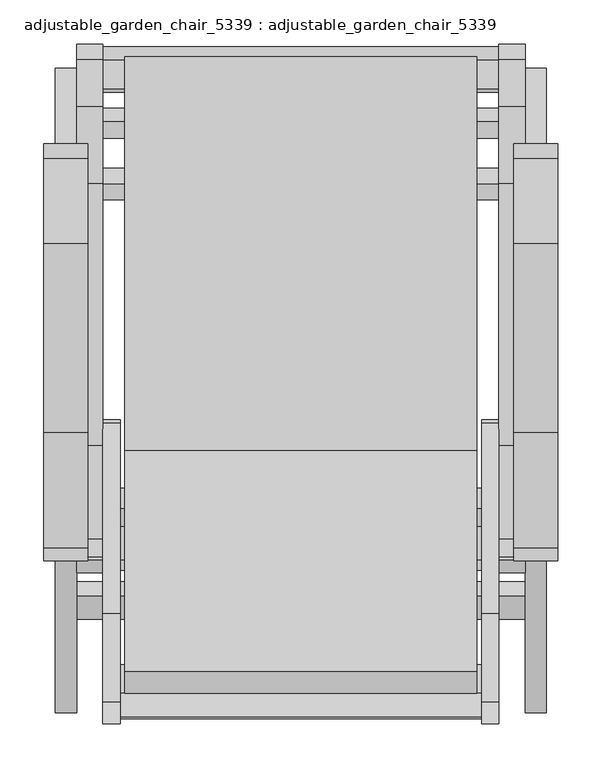
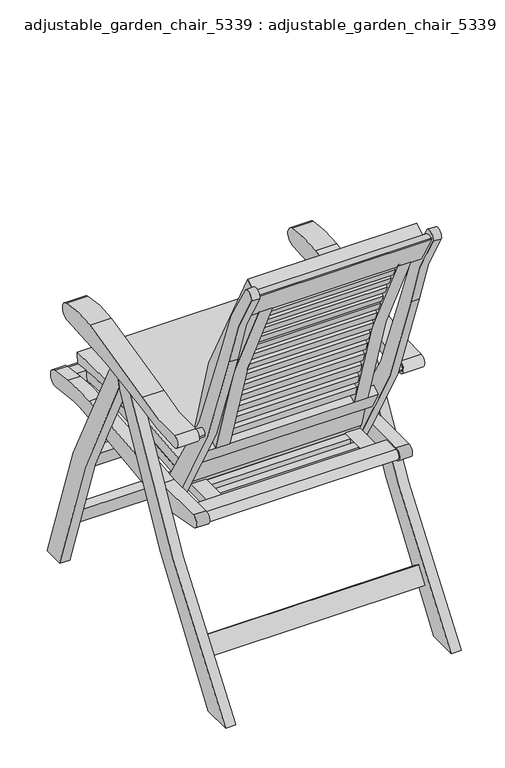
"""IFC4 building model written with IfcOpenShell, lengths in millimetres: furniture geometry, adjustable_garden_chair_5339 : adjustable_garden_chair_5339."""

from ifc_helpers import new_model, si_unit, point, frame, frame_2d, origin, place, context, project, spatial, polyline, circle_curve, trimmed, segment, composite_curve, outline, extrude, source, transform, mapped, element, save


def adjustable_garden_chair_5339_adjustable_garden_chair_5339_fbaf4b35(model_context):
    return source(origin(), model_context, "Body", "SweptSolid", [
        extrude(outline(composite_curve([segment(trimmed(circle_curve(frame_2d((343.645132, -510.0114028)), 1212.8355828), [point((-43.4212159, 639.4014009))], [point((170.6132595, 690.417738))], False, "CARTESIAN"), True, "CONTINUOUS"), segment(trimmed(circle_curve(frame_2d((209.9588085, 417.4533248)), 275.7855019), [point((170.6132595, 690.417738))], [point((267.5231892, 687.1642537))], False, "CARTESIAN"), True, "CONTINUOUS"), segment(trimmed(circle_curve(frame_2d((263.0738268, 666.3173055)), 21.3164742), [point((267.5231892, 687.1642537))], [point((263.2618422, 645.0016605))], False, "CARTESIAN"), True, "CONTINUOUS"), segment(trimmed(circle_curve(frame_2d((275.8190799, -778.6351578)), 1423.692198), [point((263.2618422, 645.0016605))], [point((-39.8991519, 609.6088672))], True, "CARTESIAN"), True, "CONTINUOUS"), segment(trimmed(circle_curve(frame_2d((-181.4513875, 1232.0279279)), 638.3122454), [point((-39.8991519, 609.6088672))], [point((-173.9655536, 593.7595793))], False, "CARTESIAN"), True, "CONTINUOUS"), segment(trimmed(circle_curve(frame_2d((-174.7344479, 608.5698693)), 14.8302356), [point((-173.9655536, 593.7595793))], [point((-175.5033422, 623.3801593))], False, "CARTESIAN"), True, "CONTINUOUS"), segment(trimmed(circle_curve(frame_2d((-148.1612086, 950.4320275)), 328.1928043), [point((-175.5033422, 623.3801593))], [point((-43.4212159, 639.4014009))], True, "CARTESIAN"), True, "CONTINUOUS")], self_intersect=False)), frame((242.0, 0.0, 0.0), z_axis=(1.0, 0.0, 0.0), x_axis=(0.0, 1.0, 0.0)), (0.0, 0.0, 1.0), 50.0),
        extrude(outline(composite_curve([segment(trimmed(circle_curve(frame_2d((343.645132, -510.0114028)), 1212.8355828), [point((-43.4212159, 639.4014009))], [point((170.6132595, 690.417738))], False, "CARTESIAN"), True, "CONTINUOUS"), segment(trimmed(circle_curve(frame_2d((209.9588085, 417.4533248)), 275.7855019), [point((170.6132595, 690.417738))], [point((267.5231892, 687.1642537))], False, "CARTESIAN"), True, "CONTINUOUS"), segment(trimmed(circle_curve(frame_2d((263.0738268, 666.3173055)), 21.3164742), [point((267.5231892, 687.1642537))], [point((263.2618422, 645.0016605))], False, "CARTESIAN"), True, "CONTINUOUS"), segment(trimmed(circle_curve(frame_2d((275.8190799, -778.6351578)), 1423.692198), [point((263.2618422, 645.0016605))], [point((-39.8991519, 609.6088672))], True, "CARTESIAN"), True, "CONTINUOUS"), segment(trimmed(circle_curve(frame_2d((-181.4513875, 1232.0279279)), 638.3122454), [point((-39.8991519, 609.6088672))], [point((-173.9655536, 593.7595793))], False, "CARTESIAN"), True, "CONTINUOUS"), segment(trimmed(circle_curve(frame_2d((-174.7344479, 608.5698693)), 14.8302356), [point((-173.9655536, 593.7595793))], [point((-175.5033422, 623.3801593))], False, "CARTESIAN"), True, "CONTINUOUS"), segment(trimmed(circle_curve(frame_2d((-148.1612086, 950.4320275)), 328.1928043), [point((-175.5033422, 623.3801593))], [point((-43.4212159, 639.4014009))], True, "CARTESIAN"), True, "CONTINUOUS")], self_intersect=False)), frame((-292.0, 0.0, 0.0), z_axis=(1.0, 0.0, 0.0), x_axis=(0.0, 1.0, 0.0)), (0.0, 0.0, 1.0), 50.0),
        extrude(outline(polyline([(0.0, 20.0), (295.0, 20.0), (295.0, 0.0), (0.0, 0.0), (0.0, 20.0)])), frame((147.5, -137.5882722, 568.6800749), z_axis=(0.0, -0.2533030270582979, 0.9673869838296892), x_axis=(-1.0, 0.0, 0.0)), (0.0, 0.0, 1.0), 20.0),
        extrude(outline(polyline([(0.0, 20.0), (295.0, 20.0), (295.0, 0.0), (0.0, 0.0), (0.0, 20.0)])), frame((147.5, -147.2074959, 603.5678435), z_axis=(0.0, -0.2719015325291372, 0.9623250784471465), x_axis=(-1.0, 0.0, 0.0)), (0.0, 0.0, 1.0), 20.0),
        extrude(outline(polyline([(0.0, 19.9999999), (295.0, 19.9999999), (295.0, 0.0), (0.0, 0.0), (0.0, 19.9999999)])), frame((147.5, -157.4973647, 638.2637288), z_axis=(0.0, -0.2903990191599495, 0.9569056430343272), x_axis=(-1.0, 0.0, 0.0)), (0.0, 0.0, 1.0), 20.0),
        extrude(outline(polyline([(0.0, 20.0000001), (295.0, 20.0000001), (295.0, 0.0), (0.0, 0.0), (0.0, 20.0000001)])), frame((147.5, -168.4540556, 672.7548405), z_axis=(0.0, -0.30878861462961876, 0.9511306910593943), x_axis=(-1.0, 0.0, 0.0)), (0.0, 0.0, 1.0), 20.0),
        extrude(outline(polyline([(0.0, 20.0), (295.0, 20.0), (295.0, 0.0), (0.0, 0.0), (0.0, 20.0)])), frame((147.5, -180.073498, 707.028364), z_axis=(0.0, -0.3270634867015429, 0.9450023680746149), x_axis=(-1.0, 0.0, 0.0)), (0.0, 0.0, 1.0), 20.0),
        extrude(outline(polyline([(0.0, 20.0), (295.0, 20.0), (295.0, 0.0), (0.0, 0.0), (0.0, 20.0)])), frame((147.5, -192.3513749, 741.071566), z_axis=(0.0, -0.3452168457619835, 0.9385229509192341), x_axis=(-1.0, 0.0, 0.0)), (0.0, 0.0, 1.0), 20.0),
        extrude(outline(polyline([(0.0, 20.0), (295.0, 20.0), (295.0, 0.0), (0.0, 0.0), (0.0, 20.0)])), frame((147.5, -205.2831247, 774.8717983), z_axis=(0.0, -0.3632419473426192, 0.9316948468735576), x_axis=(-1.0, 0.0, 0.0)), (0.0, 0.0, 1.0), 20.0),
        extrude(outline(polyline([(0.0, 20.0), (295.0, 20.0), (295.0, 0.0), (0.0, 0.0), (0.0, 20.0)])), frame((147.5, -218.863943, 808.4165033), z_axis=(0.0, -0.38113209462627146, 0.9245205927645911), x_axis=(-1.0, 0.0, 0.0)), (0.0, 0.0, 1.0), 20.0),
        extrude(outline(polyline([(0.0, 20.0000001), (295.0, 20.0000001), (295.0, 0.0), (0.0, 0.0), (0.0, 20.0000001)])), frame((147.5, -233.088784, 841.6932183), z_axis=(0.0, -0.39888064093497316, 0.9170028540235331), x_axis=(-1.0, 0.0, 0.0)), (0.0, 0.0, 1.0), 20.0),
        extrude(outline(polyline([(0.0, 20.0), (295.0, 20.0), (295.0, 0.0), (0.0, 0.0), (0.0, 20.0)])), frame((147.5, -244.4121321, 867.0975304), z_axis=(0.0, -0.4164809921993657, 0.9091444236955051), x_axis=(-1.0, 0.0, 0.0)), (0.0, 0.0, 1.0), 20.0),
        extrude(outline(polyline([(0.0, 20.0), (295.0, 20.0), (295.0, 0.0), (0.0, 0.0), (0.0, 20.0)])), frame((147.5, -259.9089267, 899.8012797), z_axis=(0.0, -0.43392660940863675, 0.9009482214018321), x_axis=(-1.0, 0.0, 0.0)), (0.0, 0.0, 1.0), 20.0),
        extrude(outline(polyline([(0.0, 20.0000001), (295.0, 20.0000001), (295.0, 0.0), (0.0, 0.0), (0.0, 20.0000001)])), frame((147.5, -276.0331794, 932.2002663), z_axis=(0.0, -0.4512110110398427, 0.892417292255368), x_axis=(-1.0, 0.0, 0.0)), (0.0, 0.0, 1.0), 20.0),
        extrude(outline(polyline([(0.0, 20.0), (295.0, 20.0), (295.0, 0.0), (0.0, 0.0), (0.0, 20.0)])), frame((147.5, -292.7788997, 964.2824531), z_axis=(0.0, -0.4683277754660565, 0.8835548057291156), x_axis=(-1.0, 0.0, 0.0)), (0.0, 0.0, 1.0), 20.0),
        extrude(outline(composite_curve([segment(trimmed(circle_curve(frame_2d((-1820.3447932, 139.3902819)), 1716.607402), [point((-150.6635772, 538.0199468))], [point((-330.8196286, 992.6521155))], True, "CARTESIAN"), True, "CONTINUOUS"), segment(polyline([(-330.8196286, 992.6521155), (-311.3178699, 1002.7482844)]), True, "CONTINUOUS"), segment(trimmed(circle_curve(frame_2d((-1820.3447932, 139.3902819)), 1738.5480424), [point((-311.3178699, 1002.7482844))], [point((-130.6557697, 548.6582867))], False, "CARTESIAN"), True, "CONTINUOUS"), segment(polyline([(-130.6557697, 548.6582867), (-150.6635772, 538.0199468)]), True, "CONTINUOUS")], self_intersect=False)), frame((147.5, 0.0, 0.0), z_axis=(1.0, 0.0, 0.0), x_axis=(0.0, 1.0, 0.0)), (0.0, 0.0, 1.0), 32.5),
        extrude(outline(composite_curve([segment(trimmed(circle_curve(frame_2d((-1820.3447932, 139.3902819)), 1716.607402), [point((-150.6635772, 538.0199468))], [point((-330.8196286, 992.6521155))], True, "CARTESIAN"), True, "CONTINUOUS"), segment(polyline([(-330.8196286, 992.6521155), (-311.3178699, 1002.7482844)]), True, "CONTINUOUS"), segment(trimmed(circle_curve(frame_2d((-1820.3447932, 139.3902819)), 1738.5480424), [point((-311.3178699, 1002.7482844))], [point((-130.6557697, 548.6582867))], False, "CARTESIAN"), True, "CONTINUOUS"), segment(polyline([(-130.6557697, 548.6582867), (-150.6635772, 538.0199468)]), True, "CONTINUOUS")], self_intersect=False)), frame((-180.0, 0.0, 0.0), z_axis=(1.0, 0.0, 0.0), x_axis=(0.0, 1.0, 0.0)), (0.0, 0.0, 1.0), 32.5),
        extrude(outline(polyline([(0.0, 22.0), (411.0, 22.0), (411.0, 0.0), (0.0, 0.0), (0.0, 22.0)])), frame((205.5, -107.1821916, 504.5109071), z_axis=(0.0, -0.46947156278588487, 0.8829475928589302), x_axis=(-1.0, 0.0, 0.0)), (0.0, 0.0, 1.0), 50.0),
        extrude(outline(composite_curve([segment(polyline([(-369.2008252, 1058.8126612), (-367.4620723, 1059.800962)]), True, "CONTINUOUS"), segment(trimmed(circle_curve(frame_2d((-357.5790638, 1042.4134336)), 20.0), [point((-367.4620723, 1059.800962))], [point((-340.1915354, 1052.2964421))], False, "CARTESIAN"), True, "CONTINUOUS"), segment(polyline([(-340.1915354, 1052.2964421), (-308.0717579, 995.7869748), (-327.1980391, 984.9156655), (-369.2008252, 1058.8126612)]), True, "CONTINUOUS")], self_intersect=False)), frame((-205.5, 0.0, 0.0), z_axis=(1.0, 0.0, 0.0), x_axis=(0.0, 1.0, 0.0)), (0.0, 0.0, 1.0), 411.0),
        extrude(outline(composite_curve([segment(trimmed(circle_curve(frame_2d((-878.1941568, 714.0152031)), 609.3375862), [point((-284.5644955, 851.478359))], [point((-374.7410315, 1057.2749365))], True, "CARTESIAN"), True, "CONTINUOUS"), segment(trimmed(circle_curve(frame_2d((-359.5368178, 1059.9113552)), 15.4310991), [point((-374.7410315, 1057.2749365))], [point((-350.3591165, 1072.3165403))], False, "CARTESIAN"), True, "CONTINUOUS"), segment(trimmed(circle_curve(frame_2d((-939.3593126, 662.5924291)), 717.4922148), [point((-350.3591165, 1072.3165403))], [point((-249.8732333, 861.0968995))], False, "CARTESIAN"), True, "CONTINUOUS"), segment(trimmed(circle_curve(frame_2d((1197.5178376, 1277.8037867)), 1506.1824398), [point((-249.8732333, 861.0968995))], [point((-33.307137, 409.6704883))], True, "CARTESIAN"), True, "CONTINUOUS"), segment(trimmed(circle_curve(frame_2d((-52.4582417, 396.9808098)), 22.9737405), [point((-33.307137, 409.6704883))], [point((-71.610087, 384.292249))], False, "CARTESIAN"), True, "CONTINUOUS"), segment(trimmed(circle_curve(frame_2d((1314.5285091, 1298.2546646)), 1660.3335522), [point((-71.610087, 384.292249))], [point((-284.5644955, 851.478359))], False, "CARTESIAN"), True, "CONTINUOUS")], self_intersect=False)), frame((205.5, 0.0, 0.0), z_axis=(1.0, 0.0, 0.0), x_axis=(0.0, 1.0, 0.0)), (0.0, 0.0, 1.0), 19.5),
        extrude(outline(composite_curve([segment(trimmed(circle_curve(frame_2d((-878.1941568, 714.0152031)), 609.3375862), [point((-284.5644955, 851.478359))], [point((-374.7410315, 1057.2749365))], True, "CARTESIAN"), True, "CONTINUOUS"), segment(trimmed(circle_curve(frame_2d((-359.53684, 1059.9114029)), 15.4310853), [point((-374.7410315, 1057.2749365))], [point((-350.3591359, 1072.3165688))], False, "CARTESIAN"), True, "CONTINUOUS"), segment(trimmed(circle_curve(frame_2d((-939.3594209, 662.5923787)), 717.4923328), [point((-350.3591359, 1072.3165688))], [point((-249.8732333, 861.0968995))], False, "CARTESIAN"), True, "CONTINUOUS"), segment(trimmed(circle_curve(frame_2d((1197.5180648, 1277.8038927)), 1506.1826875), [point((-249.8732333, 861.0968995))], [point((-33.3071379, 409.6704879))], True, "CARTESIAN"), True, "CONTINUOUS"), segment(trimmed(circle_curve(frame_2d((-52.4582393, 396.9808109)), 22.973737), [point((-33.3071379, 409.6704879))], [point((-71.6100814, 384.2922516))], False, "CARTESIAN"), True, "CONTINUOUS"), segment(trimmed(circle_curve(frame_2d((1314.5305815, 1298.2556309)), 1660.3358082), [point((-71.6100814, 384.2922516))], [point((-284.5644955, 851.478359))], False, "CARTESIAN"), True, "CONTINUOUS")], self_intersect=False)), frame((-225.0, 0.0, 0.0), z_axis=(1.0, 0.0, 0.0), x_axis=(0.0, 1.0, 0.0)), (0.0, 0.0, 1.0), 19.5),
        extrude(outline(composite_curve([segment(trimmed(circle_curve(frame_2d((73.4314655, 579.8735129)), 50.1264871), [point((83.9411598, 628.8858688))], [point((115.5965217, 606.9802048))], False, "CARTESIAN"), True, "CONTINUOUS"), segment(trimmed(circle_curve(frame_2d((-2141.3775013, -695.7889548)), 2605.9814319), [point((115.5965217, 606.9802048))], [point((370.0, 0.0))], False, "CARTESIAN"), True, "CONTINUOUS"), segment(polyline([(370.0, 0.0), (318.4314655, 0.0)]), True, "CONTINUOUS"), segment(trimmed(circle_curve(frame_2d((-2150.5800409, -679.3988459)), 2560.78125), [point((318.4314655, 0.0))], [point((73.4314655, 590.0))], True, "CARTESIAN"), True, "CONTINUOUS"), segment(polyline([(73.4314655, 590.0), (83.9411598, 628.8858688)]), True, "CONTINUOUS")], self_intersect=False)), frame((255.0, 0.0, 0.0), z_axis=(1.0, 0.0, 0.0), x_axis=(0.0, 1.0, 0.0)), (0.0, 0.0, 1.0), 24.0),
        extrude(outline(composite_curve([segment(trimmed(circle_curve(frame_2d((-2678.9114955, 1935.6417432)), 3018.90625), [point((-362.21428, 0.0))], [point((30.5273572, 604.2004001))], True, "CARTESIAN"), True, "CONTINUOUS"), segment(trimmed(circle_curve(frame_2d((72.4622197, 583.5932512)), 46.7245896), [point((30.5273572, 604.2004001))], [point((83.9411598, 628.8858688))], False, "CARTESIAN"), True, "CONTINUOUS"), segment(polyline([(83.9411598, 628.8858688), (73.4314655, 590.0)]), True, "CONTINUOUS"), segment(trimmed(circle_curve(frame_2d((-2658.8629803, 1872.415208)), 3018.28125), [point((73.4314655, 590.0))], [point((-291.5685345, 0.0))], False, "CARTESIAN"), True, "CONTINUOUS"), segment(polyline([(-291.5685345, 0.0), (-362.21428, 0.0)]), True, "CONTINUOUS")], self_intersect=False)), frame((255.0, 0.0, 0.0), z_axis=(1.0, 0.0, 0.0), x_axis=(0.0, 1.0, 0.0)), (0.0, 0.0, 1.0), 24.0),
        extrude(outline(composite_curve([segment(trimmed(circle_curve(frame_2d((73.4314655, 579.8735129)), 50.1264871), [point((83.9411598, 628.8858688))], [point((115.5965217, 606.9802048))], False, "CARTESIAN"), True, "CONTINUOUS"), segment(trimmed(circle_curve(frame_2d((-2141.3775013, -695.7889548)), 2605.9814319), [point((115.5965217, 606.9802048))], [point((370.0, 0.0))], False, "CARTESIAN"), True, "CONTINUOUS"), segment(polyline([(370.0, 0.0), (318.4314655, 0.0)]), True, "CONTINUOUS"), segment(trimmed(circle_curve(frame_2d((-2150.5800409, -679.3988459)), 2560.78125), [point((318.4314655, 0.0))], [point((73.4314655, 590.0))], True, "CARTESIAN"), True, "CONTINUOUS"), segment(polyline([(73.4314655, 590.0), (83.9411598, 628.8858688)]), True, "CONTINUOUS")], self_intersect=False)), frame((-279.0, 0.0, 0.0), z_axis=(1.0, 0.0, 0.0), x_axis=(0.0, 1.0, 0.0)), (0.0, 0.0, 1.0), 24.0),
        extrude(outline(composite_curve([segment(trimmed(circle_curve(frame_2d((-2678.9114955, 1935.6417432)), 3018.90625), [point((-362.21428, 0.0))], [point((30.5273572, 604.2004001))], True, "CARTESIAN"), True, "CONTINUOUS"), segment(trimmed(circle_curve(frame_2d((72.4622197, 583.5932512)), 46.7245896), [point((30.5273572, 604.2004001))], [point((83.9411598, 628.8858688))], False, "CARTESIAN"), True, "CONTINUOUS"), segment(polyline([(83.9411598, 628.8858688), (73.4314655, 590.0)]), True, "CONTINUOUS"), segment(trimmed(circle_curve(frame_2d((-2658.8629803, 1872.415208)), 3018.28125), [point((73.4314655, 590.0))], [point((-291.5685345, 0.0))], False, "CARTESIAN"), True, "CONTINUOUS"), segment(polyline([(-291.5685345, 0.0), (-362.21428, 0.0)]), True, "CONTINUOUS")], self_intersect=False)), frame((-279.0, 0.0, 0.0), z_axis=(1.0, 0.0, 0.0), x_axis=(0.0, 1.0, 0.0)), (0.0, 0.0, 1.0), 24.0),
        extrude(outline(composite_curve([segment(trimmed(circle_curve(frame_2d((274.7628361, 37.698684)), 410.0), [point((238.8791572, 446.1253746))], [point((326.8914381, 444.3712905))], False, "CARTESIAN"), True, "CONTINUOUS"), segment(polyline([(326.8914381, 444.3712905), (380.1623119, 437.5428586)]), True, "CONTINUOUS"), segment(trimmed(circle_curve(frame_2d((377.6194532, 417.7051705)), 20.0), [point((380.1623119, 437.5428586))], [point((375.0765946, 397.8674824))], False, "CARTESIAN"), True, "CONTINUOUS"), segment(polyline([(375.0765946, 397.8674824), (305.4087938, 406.7977251)]), True, "CONTINUOUS"), segment(trimmed(circle_curve(frame_2d((283.1587807, 233.217954)), 175.0), [point((305.4087938, 406.7977251))], [point((260.5570748, 406.7522817))], True, "CARTESIAN"), True, "CONTINUOUS"), segment(polyline([(260.5570748, 406.7522817), (-30.0021337, 368.908854)]), True, "CONTINUOUS"), segment(trimmed(circle_curve(frame_2d((-53.2496027, 547.4013053)), 180.0), [point((-30.0021337, 368.908854))], [point((-86.6960303, 370.5359993))], False, "CARTESIAN"), True, "CONTINUOUS"), segment(polyline([(-86.6960303, 370.5359993), (-191.0033734, 390.2612245)]), True, "CONTINUOUS"), segment(trimmed(circle_curve(frame_2d((-188.2161711, 405.0)), 15.0), [point((-191.0033734, 390.2612245))], [point((-188.2161711, 420.0))], False, "CARTESIAN"), True, "CONTINUOUS"), segment(polyline([(-188.2161711, 420.0), (-58.4788796, 420.0), (238.8791572, 446.1253746)]), True, "CONTINUOUS")], self_intersect=False)), frame((225.0, 0.0, 0.0), z_axis=(1.0, 0.0, 0.0), x_axis=(0.0, 1.0, 0.0)), (0.0, 0.0, 1.0), 30.0),
        extrude(outline(composite_curve([segment(trimmed(circle_curve(frame_2d((274.7628361, 37.698684)), 410.0), [point((238.8791572, 446.1253746))], [point((326.8914381, 444.3712905))], False, "CARTESIAN"), True, "CONTINUOUS"), segment(polyline([(326.8914381, 444.3712905), (380.1623119, 437.5428586)]), True, "CONTINUOUS"), segment(trimmed(circle_curve(frame_2d((377.6194532, 417.7051705)), 20.0), [point((380.1623119, 437.5428586))], [point((375.0765946, 397.8674824))], False, "CARTESIAN"), True, "CONTINUOUS"), segment(polyline([(375.0765946, 397.8674824), (305.4087938, 406.7977251)]), True, "CONTINUOUS"), segment(trimmed(circle_curve(frame_2d((283.1587807, 233.217954)), 175.0), [point((305.4087938, 406.7977251))], [point((260.5570748, 406.7522817))], True, "CARTESIAN"), True, "CONTINUOUS"), segment(polyline([(260.5570748, 406.7522817), (-30.0021337, 368.908854)]), True, "CONTINUOUS"), segment(trimmed(circle_curve(frame_2d((-53.2496027, 547.4013053)), 180.0), [point((-30.0021337, 368.908854))], [point((-86.6960303, 370.5359993))], False, "CARTESIAN"), True, "CONTINUOUS"), segment(polyline([(-86.6960303, 370.5359993), (-191.0033734, 390.2612245)]), True, "CONTINUOUS"), segment(trimmed(circle_curve(frame_2d((-188.2161711, 405.0)), 15.0), [point((-191.0033734, 390.2612245))], [point((-188.2161711, 420.0))], False, "CARTESIAN"), True, "CONTINUOUS"), segment(polyline([(-188.2161711, 420.0), (-58.4788796, 420.0), (238.8791572, 446.1253746)]), True, "CONTINUOUS")], self_intersect=False)), frame((-255.0, 0.0, 0.0), z_axis=(1.0, 0.0, 0.0), x_axis=(0.0, 1.0, 0.0)), (0.0, 0.0, 1.0), 30.0),
        extrude(outline(composite_curve([segment(trimmed(circle_curve(frame_2d((377.6194532, 417.7051705)), 17.0), [point((379.7808831, 434.5672054))], [point((375.4580234, 400.8431356))], False, "CARTESIAN"), True, "CONTINUOUS"), segment(polyline([(375.4580234, 400.8431356), (342.725838, 405.0388524), (347.0486977, 438.7629222), (379.7808831, 434.5672054)]), True, "CONTINUOUS")], self_intersect=False)), frame((-225.0, 0.0, 0.0), z_axis=(1.0, 0.0, 0.0), x_axis=(0.0, 1.0, 0.0)), (0.0, 0.0, 1.0), 450.0),
        extrude(outline(composite_curve([segment(polyline([(-188.2161711, 417.0), (-150.2161711, 417.0), (-150.2161711, 392.7341457), (-188.2161711, 392.7341457)]), True, "CONTINUOUS"), segment(trimmed(circle_curve(frame_2d((-188.2161711, 404.8670728)), 12.1329272), [point((-188.2161711, 392.7341457))], [point((-188.2161711, 417.0))], False, "CARTESIAN"), True, "CONTINUOUS")], self_intersect=False)), frame((-225.0, 0.0, 0.0), z_axis=(1.0, 0.0, 0.0), x_axis=(0.0, 1.0, 0.0)), (0.0, 0.0, 1.0), 450.0),
        extrude(outline(composite_curve([segment(polyline([(-58.2596561, 415.0), (239.3167631, 441.1445613)]), True, "CONTINUOUS"), segment(trimmed(circle_curve(frame_2d((274.7628361, 37.698684)), 405.0), [point((239.3167631, 441.1445613))], [point((326.2557234, 439.4118685))], False, "CARTESIAN"), True, "CONTINUOUS"), segment(polyline([(326.2557234, 439.4118685), (346.7944118, 436.7791534), (343.9972673, 414.9576964), (323.4585789, 417.5904115)]), True, "CONTINUOUS"), segment(trimmed(circle_curve(frame_2d((274.7628361, 37.698684)), 383.0), [point((323.4585789, 417.5904115))], [point((241.2422287, 419.2289828))], True, "CARTESIAN"), True, "CONTINUOUS"), segment(polyline([(241.2422287, 419.2289828), (-57.2950725, 393.0), (-150.2161711, 393.0), (-150.2161711, 415.0), (-58.2596561, 415.0)]), True, "CONTINUOUS")], self_intersect=False)), frame((-200.0, 0.0, 0.0), z_axis=(1.0, 0.0, 0.0), x_axis=(0.0, 1.0, 0.0)), (0.0, 0.0, 1.0), 35.0),
        extrude(outline(composite_curve([segment(polyline([(-58.2596561, 415.0), (239.3167631, 441.1445613)]), True, "CONTINUOUS"), segment(trimmed(circle_curve(frame_2d((274.7628361, 37.698684)), 405.0), [point((239.3167631, 441.1445613))], [point((326.2557234, 439.4118685))], False, "CARTESIAN"), True, "CONTINUOUS"), segment(polyline([(326.2557234, 439.4118685), (346.7944118, 436.7791534), (343.9972673, 414.9576964), (323.4585789, 417.5904115)]), True, "CONTINUOUS"), segment(trimmed(circle_curve(frame_2d((274.7628361, 37.698684)), 383.0), [point((323.4585789, 417.5904115))], [point((241.2422287, 419.2289828))], True, "CARTESIAN"), True, "CONTINUOUS"), segment(polyline([(241.2422287, 419.2289828), (-57.2950725, 393.0), (-150.2161711, 393.0), (-150.2161711, 415.0), (-58.2596561, 415.0)]), True, "CONTINUOUS")], self_intersect=False)), frame((165.0, 0.0, 0.0), z_axis=(1.0, 0.0, 0.0), x_axis=(0.0, 1.0, 0.0)), (0.0, 0.0, 1.0), 35.0),
        extrude(outline(polyline([(0.0, 20.0), (330.0, 20.0), (330.0, 0.0), (0.0, 0.0), (0.0, 20.0)])), frame((165.0, 329.8129674, 417.7918808), z_axis=(0.0, 0.10015135080024025, 0.9949722141511729), x_axis=(-1.0, 0.0, 0.0)), (0.0, 0.0, 1.0), 20.0),
        extrude(outline(polyline([(0.0, 20.0), (330.0, 20.0), (330.0, 0.0), (0.0, 0.0), (0.0, 20.0)])), frame((165.0, 295.940466, 420.5485593), z_axis=(0.0, 0.05430307370314669, 0.9985244995423951), x_axis=(-1.0, 0.0, 0.0)), (0.0, 0.0, 1.0), 20.0),
        extrude(outline(polyline([(0.0, 20.0), (330.0, 20.0), (330.0, 0.0), (0.0, 0.0), (0.0, 20.0)])), frame((165.0, 262.8732701, 420.9868234), z_axis=(0.0, -0.0399406917008388, 0.9992020522128938), x_axis=(-1.0, 0.0, 0.0)), (0.0, 0.0, 1.0), 20.0),
        extrude(outline(polyline([(0.0, 19.9999999), (330.0, 19.9999999), (330.0, 0.0), (0.0, 0.0), (0.0, 19.9999999)])), frame((165.0, 228.8710651, 419.149381), z_axis=(0.0, -0.0862771077257393, 0.9962711782855516), x_axis=(-1.0, 0.0, 0.0)), (0.0, 0.0, 1.0), 20.0),
        extrude(outline(polyline([(0.0, 19.9999999), (330.0, 19.9999999), (330.0, 0.0), (0.0, 0.0), (0.0, 19.9999999)])), frame((165.0, 194.005372, 416.0861402), z_axis=(0.0, -0.0862771077257393, 0.9962711782855516), x_axis=(-1.0, 0.0, 0.0)), (0.0, 0.0, 1.0), 20.0),
        extrude(outline(polyline([(0.0, 19.9999999), (330.0, 19.9999999), (330.0, 0.0), (0.0, 0.0), (0.0, 19.9999999)])), frame((165.0, 159.1396789, 413.0228993), z_axis=(0.0, -0.08627710772573936, 0.9962711782855516), x_axis=(-1.0, 0.0, 0.0)), (0.0, 0.0, 1.0), 20.0),
        extrude(outline(polyline([(0.0, 19.9999999), (330.0, 19.9999999), (330.0, 0.0), (0.0, 0.0), (0.0, 19.9999999)])), frame((165.0, 124.2739858, 409.9596584), z_axis=(0.0, -0.08627710772573943, 0.9962711782855516), x_axis=(-1.0, 0.0, 0.0)), (0.0, 0.0, 1.0), 20.0),
        extrude(outline(polyline([(0.0, 19.9999999), (330.0, 19.9999999), (330.0, 0.0), (0.0, 0.0), (0.0, 19.9999999)])), frame((165.0, 89.4082927, 406.8964175), z_axis=(0.0, -0.0862771077257394, 0.9962711782855516), x_axis=(-1.0, 0.0, 0.0)), (0.0, 0.0, 1.0), 20.0),
        extrude(outline(polyline([(0.0, 19.9999999), (330.0, 19.9999999), (330.0, 0.0), (0.0, 0.0), (0.0, 19.9999999)])), frame((165.0, 54.5425996, 403.8331766), z_axis=(0.0, -0.0862771077257394, 0.9962711782855516), x_axis=(-1.0, 0.0, 0.0)), (0.0, 0.0, 1.0), 20.0),
        extrude(outline(polyline([(0.0, 19.9999999), (330.0, 19.9999999), (330.0, 0.0), (0.0, 0.0), (0.0, 19.9999999)])), frame((165.0, 19.6769065, 400.7699358), z_axis=(0.0, -0.08627710772573942, 0.9962711782855516), x_axis=(-1.0, 0.0, 0.0)), (0.0, 0.0, 1.0), 20.0),
        extrude(outline(polyline([(0.0, 19.9999999), (330.0, 19.9999999), (330.0, 0.0), (0.0, 0.0), (0.0, 19.9999999)])), frame((165.0, -15.1887866, 397.7066949), z_axis=(0.0, -0.0862771077257394, 0.9962711782855516), x_axis=(-1.0, 0.0, 0.0)), (0.0, 0.0, 1.0), 20.0),
        extrude(outline(polyline([(0.0, 20.0), (330.0, 20.0), (330.0, 0.0), (0.0, 0.0), (0.0, 20.0)])), frame((165.0, -50.5659752, 394.1151581), z_axis=(0.0, -0.03230033547544253, 0.9994782080306573), x_axis=(-1.0, 0.0, 0.0)), (0.0, 0.0, 1.0), 20.0),
        extrude(outline(polyline([(165.0, -106.2119819), (-165.0, -106.2119819), (-165.0, -86.2119819), (165.0, -86.2119819), (165.0, -106.2119819)])), frame((0.0, 0.0, 394.1047223), z_axis=(0.0, 0.0, 1.0), x_axis=(1.0, 0.0, 0.0)), (0.0, 0.0, 1.0), 20.0),
        extrude(outline(polyline([(165.0, -141.2119819), (-165.0, -141.2119819), (-165.0, -121.2119819), (165.0, -121.2119819), (165.0, -141.2119819)])), frame((0.0, 0.0, 394.1047223), z_axis=(0.0, 0.0, 1.0), x_axis=(1.0, 0.0, 0.0)), (0.0, 0.0, 1.0), 20.0),
        extrude(outline(polyline([(0.0, 20.0), (510.0, 20.0), (510.0, 0.0), (0.0, 0.0), (0.0, 20.0)])), frame((255.0, 324.5742376, 103.4202014), z_axis=(0.0, -0.34202014332566577, 0.9396926207859095), x_axis=(-1.0, 0.0, 0.0)), (0.0, 0.0, 1.0), 45.0),
        extrude(outline(polyline([(0.0, 20.0), (510.0, 20.0), (510.0, 0.0), (0.0, 0.0), (0.0, 20.0)])), frame((255.0, -239.7030548, 94.1221475), z_axis=(0.0, 0.5877852522924797, 0.8090169943749427), x_axis=(-1.0, 0.0, 0.0)), (0.0, 0.0, 1.0), 45.0),
        extrude(outline(polyline([(0.0, 20.0), (510.0, 20.0), (510.0, 0.0), (0.0, 0.0), (0.0, 20.0)])), frame((255.0, 256.6989851, 287.857913), z_axis=(0.0, -0.3907311284892644, 0.9205048534524444), x_axis=(-1.0, 0.0, 0.0)), (0.0, 0.0, 1.0), 45.0),
        extrude(outline(composite_curve([segment(trimmed(circle_curve(frame_2d((-175.2156419, 609.0447403)), 10.0), [point((-165.2603514, 609.9892995))], [point((-185.1709323, 608.1001811))], False, "CARTESIAN"), True, "CONTINUOUS"), segment(trimmed(circle_curve(frame_2d((-175.2156419, 609.0447403)), 10.0), [point((-185.1709323, 608.1001811))], [point((-165.2603514, 609.9892995))], False, "CARTESIAN"), True, "CONTINUOUS")], self_intersect=False)), frame((-242.0, 0.0, 0.0), z_axis=(1.0, 0.0, 0.0), x_axis=(0.0, 1.0, 0.0)), (0.0, 0.0, 1.0), 17.0),
        extrude(outline(composite_curve([segment(trimmed(circle_curve(frame_2d((-175.2156419, 609.0447403)), 10.0), [point((-165.2603514, 609.9892995))], [point((-185.1709323, 608.1001811))], False, "CARTESIAN"), True, "CONTINUOUS"), segment(trimmed(circle_curve(frame_2d((-175.2156419, 609.0447403)), 10.0), [point((-185.1709323, 608.1001811))], [point((-165.2603514, 609.9892995))], False, "CARTESIAN"), True, "CONTINUOUS")], self_intersect=False)), frame((225.0, 0.0, 0.0), z_axis=(1.0, 0.0, 0.0), x_axis=(0.0, 1.0, 0.0)), (0.0, 0.0, 1.0), 17.0),
        extrude(outline(composite_curve([segment(polyline([(-83.6234956, 412.7715759), (-88.4238262, 442.3850328)]), True, "CONTINUOUS"), segment(trimmed(circle_curve(frame_2d((231.1593215, -1529.137865)), 1997.2571003), [point((-88.4238262, 442.3850328))], [point((383.0914779, 462.3320807))], False, "CARTESIAN"), True, "CONTINUOUS"), segment(polyline([(383.0914779, 462.3320807), (380.8093658, 432.4190072)]), True, "CONTINUOUS"), segment(trimmed(circle_curve(frame_2d((231.1593215, -1529.137865)), 1967.2571003), [point((380.8093658, 432.4190072))], [point((-83.6234956, 412.7715759))], True, "CARTESIAN"), True, "CONTINUOUS")], self_intersect=False)), frame((-200.0, 0.0, 0.0), z_axis=(1.0, 0.0, 0.0), x_axis=(0.0, 1.0, 0.0)), (0.0, 0.0, 1.0), 400.0),
        extrude(outline(composite_curve([segment(polyline([(-340.9641484, 1052.5869946), (-315.8143742, 1068.9420811)]), True, "CONTINUOUS"), segment(trimmed(circle_curve(frame_2d((-1798.4338397, 104.7835367)), 1768.5480424), [point((-315.8143742, 1068.9420811))], [point((-60.2814137, 431.2622072))], False, "CARTESIAN"), True, "CONTINUOUS"), segment(polyline([(-60.2814137, 431.2622072), (-89.7658108, 425.7241274)]), True, "CONTINUOUS"), segment(trimmed(circle_curve(frame_2d((-1798.4338397, 104.7835367)), 1738.5480424), [point((-89.7658108, 425.7241274))], [point((-340.9641484, 1052.5869946))], True, "CARTESIAN"), True, "CONTINUOUS")], self_intersect=False)), frame((-200.0, 0.0, 0.0), z_axis=(1.0, 0.0, 0.0), x_axis=(0.0, 1.0, 0.0)), (0.0, 0.0, 1.0), 400.0),
    ])


if __name__ == "__main__":
    model = new_model("IFC4")
    model_context = context("Model", 3, world=origin())
    ifc_project = project(units=[si_unit("LENGTHUNIT", "METRE", prefix="MILLI")], contexts=[model_context])
    site = spatial("IfcSite", under=ifc_project)
    building = spatial("IfcBuilding", under=site)
    placement = place(None, origin())
    adjustable_garden_chair_5339_adjustable_garden_chair_5339_shape = adjustable_garden_chair_5339_adjustable_garden_chair_5339_fbaf4b35(model_context)
    element("IfcFurniture", 1, ObjectType="adjustable_garden_chair_5339 : adjustable_garden_chair_5339", at=placement, inside=building, context=model_context, shape_type="MappedRepresentation", body=[
        mapped(adjustable_garden_chair_5339_adjustable_garden_chair_5339_shape, transform((0.0, 0.0, 0.0), x_axis=(1.0, 0.0, 0.0), y_axis=(0.0, 1.0, 0.0), z_axis=(0.0, 0.0, 1.0))),
    ])
    save(model, "model.ifc")

# Revit data of these elements
# Type "adjustable_garden_chair_5339 : adjustable_garden_chair_5339"
#   URL = "www.revitlog.nl"
#   diepte = 2' - 7.49606"
#   corner back [instance default] = 120.00°
#   breedte = 1' - 8.07874"
#   kussen visible [instance default] = yes
#   stoel = hout
#   Default Elevation = 0
# Element 1 (IfcFurniture, "adjustable_garden_chair_5339 : adjustable_garden_chair_5339")
#   Materials on its faces: "hout"
# Materials
#   "hout": class "Wood", colour RGB 140 61 26, transparency 0
